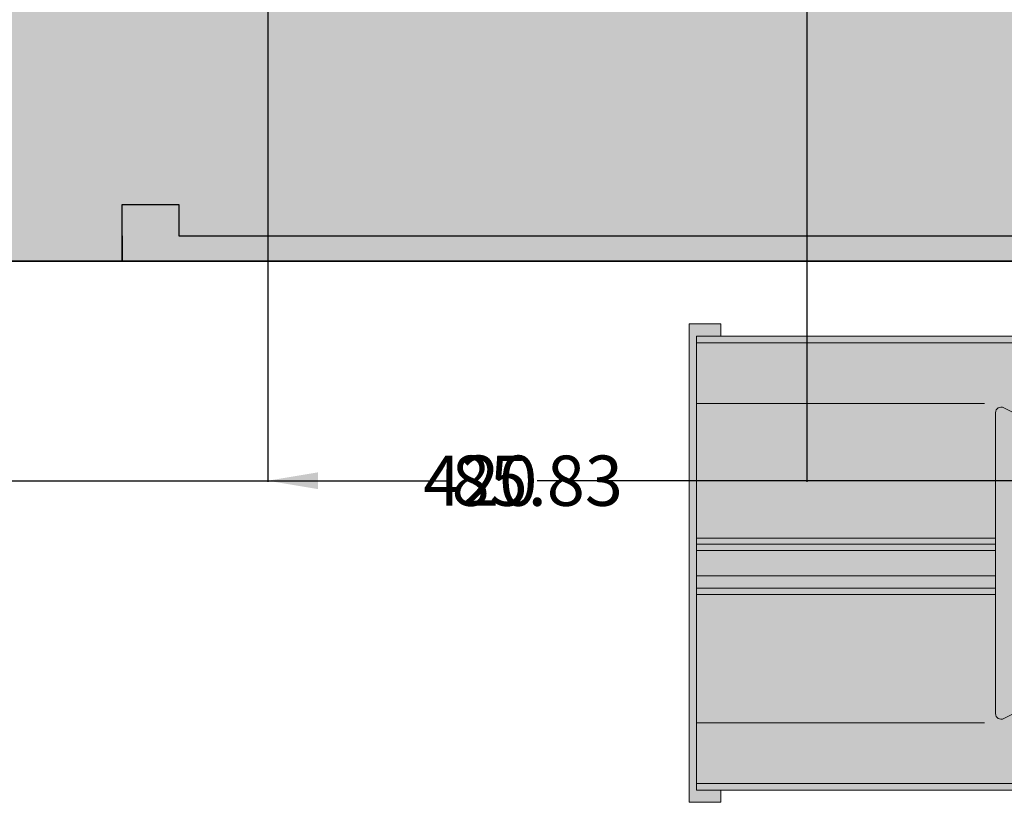
# Model space of a CAD drawing. Units: inches. Extents: x 389 to 971, y 148 to 870.
# Tile 3 of 14: x 565 to 722, y 148 to 273. Entities that reach past the tile are written whole.
import ezdxf

# ---------------------------------------------------------------- set-up
doc = ezdxf.new("R2010")
doc.units = ezdxf.units.IN
doc.header["$MEASUREMENT"] = 0
for name, color, linetype, lineweight in [('A-ANNO-DIMS', 2, 'Continuous', 18), ('C-PROP', 7, 'Continuous', 35), ('C-VEHI', 8, 'Continuous', 13), ('L-GATE', 4, 'Continuous', 25), ('L-GRND-BASE-PATT', 8, 'Continuous', 13), ('L-WALL', 7, 'Continuous', 30)]:
    doc.layers.add(name, color=color, linetype=linetype, lineweight=lineweight)
for name, color, linetype, lineweight, true_color in [('A-WALL-PATT', 18, 'Continuous', 13, 0x000000), ('C-VEHI-PATT', 18, 'Continuous', 13, 0x000000), ('L-GRND-PATT', 39, 'Continuous', 13, 0x603913), ('L-WALL-PATT', 18, 'Continuous', 13, 0x000000)]:
    doc.layers.add(name, color=color, linetype=linetype, lineweight=lineweight, true_color=true_color)
doc.styles.get("Standard").update_dxf_attribs({"font": 'arial.ttf'})
doc.dimstyles.get("Standard").update_dxf_attribs({"dimtxt": 8, "dimasz": 8, "dimexe": 0.18, "dimexo": 0.0625, "dimgap": 0.09, "dimtad": 0, "dimtih": 1, "dimtoh": 1, "dimdec": 0, "dimzin": 0, "dimdsep": 46, "dimlunit": 3, "dimtxsty": 'Standard', "dimcen": 0.09, "dimadec": 0, "dimazin": 0, "dimtfac": 1, "dimtdec": 0, "dimtofl": 0, "dimtmove": 0, "dimatfit": 3, "dimfxl": 1, "dimtolj": 1, "dimtzin": 0, "dimarcsym": 0})

# ---------------------------------------------------------------- blocks, each defined once
blk = doc.blocks.new('*U17')
for p, q in [((1.28, 38.87), (175.66, 38.87)), ((1.28, 28.15), (52.13, 28.15)), ((1.28, -28.15), (52.13, -28.15)), ((1.28, -38.87), (175.66, -38.87))]:
    blk.add_line(p, q)
for points in [[(5.57, 40.01), (5.57, 42.18), (0, 42.18), (0, -42.18), (5.57, -42.18), (5.57, -40.01), (1.28, -40.01), (1.28, 40.01)], [(1.28, 40.01), (175.66, 40.01), (175.66, -40.01), (1.28, -40.01)]]:
    blk.add_lwpolyline(points, close=True)
blk.add_lwpolyline([(55.49, 27.42), (68.59, 20.89, -0.284287), (69.14, 19.99), (69.14, -19.99, -0.284287), (68.59, -20.89), (55.49, -27.42, -0.557284), (54.05, -26.53), (54.05, 26.53, -0.557284)], format="xyb", close=True)
blk = doc.blocks.new('*D44')
at = {"layer": 'A-ANNO-DIMS', "color": 0, "lineweight": -2, "transparency": 16777216}
for p, q in [((428.22, 234.58), (428.22, 199.5)), ((848.22, 234.58), (848.22, 199.5)), ((436.22, 199.68), (629.14, 199.68)), ((840.22, 199.68), (647.29, 199.68))]:
    blk.add_line(p, q, dxfattribs=at)
at = {"layer": 'A-ANNO-DIMS', "color": 0, "transparency": 16777216}
for points in [[(436.22, 201.01), (436.22, 198.34), (428.22, 199.68)], [(840.22, 201.01), (840.22, 198.34), (848.22, 199.68)]]:
    blk.add_solid(points, dxfattribs=at)
at = {"layer": 'Defpoints', "color": 0, "transparency": 16777216}
for p in [(428.22, 234.64), (848.22, 234.64), (848.22, 199.68)]:
    blk.add_point(p, dxfattribs=at)
at = {"layer": 'A-ANNO-DIMS', "color": 0, "transparency": 16777216, "insert": (638.22, 199.68), "char_height": 8, "attachment_point": 5}
blk.add_mtext('\\A1;420', dxfattribs=at)
blk = doc.blocks.new('*D50')
at = {"layer": 'A-ANNO-DIMS', "color": 0, "lineweight": -2, "transparency": 16777216}
for p, q in [((604.39, 294.58), (604.39, 199.5)), ((690.22, 294.58), (690.22, 199.5)), ((612.39, 199.68), (633.71, 199.68)), ((682.22, 199.68), (660.89, 199.68))]:
    blk.add_line(p, q, dxfattribs=at)
at = {"layer": 'A-ANNO-DIMS', "color": 0, "transparency": 16777216}
for points in [[(612.39, 201.01), (612.39, 198.34), (604.39, 199.68)], [(682.22, 201.01), (682.22, 198.34), (690.22, 199.68)]]:
    blk.add_solid(points, dxfattribs=at)
at = {"layer": 'Defpoints', "color": 0, "transparency": 16777216}
for p in [(604.39, 294.64), (690.22, 294.64), (690.22, 199.68)]:
    blk.add_point(p, dxfattribs=at)
at = {"layer": 'A-ANNO-DIMS', "color": 0, "transparency": 16777216, "insert": (647.3, 199.68), "char_height": 8, "attachment_point": 5}
blk.add_mtext('\\A1;85.83', dxfattribs=at)

msp = doc.modelspace()

# ---------------------------------------------------------------- hatches: boundary and pattern name
at = {"layer": 'A-WALL-PATT'}
h = msp.add_hatch(color=256, dxfattribs=at)
h.dxf.hatch_style = 1
h.paths.add_polyline_path([(432.216, 434.6445), (436.3673, 434.6445), (436.3673, 443.6445), (432.216, 443.6445), (432.216, 830.6445), (746.216, 830.6445), (746.216, 823.8175), (755.216, 823.8175), (755.216, 825.6445), (839.216, 825.6445), (839.216, 803.5176), (839.216, 741.6445), (755.216, 741.6445), (755.216, 748.4596), (755.1859, 748.4596), (750.716, 748.4596), (746.216, 748.4596), (746.216, 732.6445), (839.216, 732.6445), (839.216, 600.6445), (708.5171, 600.6445), (708.5171, 596.1445), (708.5171, 591.6445), (794.216, 591.6445), (794.216, 587.4291), (803.216, 587.4291), (803.216, 591.6445), (839.216, 591.6445), (839.216, 466.6012), (803.216, 466.6012), (803.216, 471.0309), (794.216, 471.0309), (794.216, 466.6012), (784.6145, 466.6012), (784.6145, 457.6012), (839.216, 457.6012), (839.216, 447.6445), (839.216, 294.6445), (810.0514, 294.6445), (810.0514, 285.6445), (839.216, 285.6445), (839.216, 238.6445), (590.216, 238.6445), (590.216, 234.6445), (848.216, 234.6445), (848.216, 834.6445), (428.216, 834.6445), (428.216, 234.6445), (437.216, 234.6445), (437.216, 243.6445), (432.216, 243.6445)])
at = {"layer": 'C-VEHI-PATT'}
h = msp.add_hatch(color=256, dxfattribs=at)
h.dxf.hatch_style = 1
h.paths.add_polyline_path([(720.2545, 210.4982), (720.2545, 162.6111, 0.55728405), (721.56, 161.8036), (733.3797, 167.7021, 0.28428722), (733.8792, 168.5096), (733.8792, 204.5997, 0.28428722), (733.3797, 205.4073), (721.56, 211.3058, 0.55728405)], flags=16)
h.paths.add_polyline_path([(672.6289, 151.4772), (723.0515, 151.4772), (723.0515, 157.3254), (736.2011, 165.949, -0.08657677), (736.9651, 166.0823), (754.137, 166.0823, -0.22787473), (755.899, 165.2353), (759.6746, 157.5735), (759.6746, 151.4772), (830.0078, 151.4772), (830.0078, 221.6321), (759.6746, 221.6321), (759.6746, 215.5358), (755.899, 207.8741, -0.22787473), (754.137, 207.0271), (736.9651, 207.0271, -0.08657677), (736.2011, 207.1603), (723.0515, 215.784), (723.0515, 221.6321), (672.6289, 221.6321)])
h.paths.add_polyline_path([(672.6289, 150.445), (676.5048, 150.445), (676.5048, 148.491), (671.4773, 148.491), (671.4773, 224.6184), (676.5048, 224.6184), (676.5048, 222.6644), (672.6289, 222.6644)])
h.paths.add_polyline_path([(735.9785, 205.941), (818.9627, 205.941), (818.9627, 167.1683), (735.9785, 167.1683)], flags=16)
h.paths.add_polyline_path([(727.5014, 158.6254), (736.5823, 164.5807, -0.14613934), (737.0772, 164.7285), (753.9813, 164.7285, -0.29765964), (754.8077, 164.1887), (757.2923, 158.5274, -0.54123619), (757.0857, 158.2111), (727.6252, 158.2111, -0.74498852)], flags=17)
h.paths.add_polyline_path([(727.5014, 214.4839, -0.74498852), (727.6252, 214.8982), (757.0857, 214.8982, -0.54123619), (757.2923, 214.5819), (754.8077, 208.9206, -0.29765964), (753.9813, 208.3808), (737.0772, 208.3808, -0.14613934), (736.5823, 208.5286)], flags=17)
h = msp.add_hatch(color=256, dxfattribs=at)
h.dxf.hatch_style = 1
h.paths.add_polyline_path([(671.4773, 224.6184), (671.4773, 148.491), (676.5048, 148.491), (676.5048, 150.445), (672.6289, 150.445), (672.6289, 222.6644), (676.5048, 222.6644), (676.5048, 224.6184)])
h = msp.add_hatch(color=256, dxfattribs=at)
h.dxf.hatch_style = 1
h.paths.add_polyline_path([(672.6289, 184.5547), (672.6289, 151.4772), (723.0515, 151.4772), (723.0515, 157.3254), (736.2011, 165.949, -0.08657677), (736.9651, 166.0823), (754.137, 166.0823, -0.22787473), (755.899, 165.2353), (759.6746, 157.5735), (759.6746, 151.4772), (830.0078, 151.4772), (830.0078, 221.6321), (759.6746, 221.6321), (759.6746, 215.5358), (755.899, 207.8741, -0.22787473), (754.137, 207.0271), (736.9651, 207.0271, -0.08657677), (736.2011, 207.1603), (723.0515, 215.784), (723.0515, 221.6321), (672.6289, 221.6321), (672.6289, 188.5547), (720.2545, 188.5547), (720.2545, 210.4982, -0.55728405), (721.56, 211.3058), (733.3797, 205.4073, -0.28428722), (733.8792, 204.5997), (733.8792, 168.5096, -0.28428722), (733.3797, 167.7021), (721.56, 161.8036, -0.55728405), (720.2545, 162.6111), (720.2545, 184.5547)], flags=17)
h.paths.add_polyline_path([(672.6289, 151.4772), (723.0515, 151.4772), (723.0515, 157.3254), (736.2011, 165.949, -0.08657677), (736.9651, 166.0823), (754.137, 166.0823, -0.22787473), (755.899, 165.2353), (759.6746, 157.5735), (759.6746, 151.4772), (830.0078, 151.4772), (830.0078, 221.6321), (759.6746, 221.6321), (759.6746, 215.5358), (755.899, 207.8741, -0.22787473), (754.137, 207.0271), (736.9651, 207.0271, -0.08657677), (736.2011, 207.1603), (723.0515, 215.784), (723.0515, 221.6321), (672.6289, 221.6321)], flags=17)
h.paths.add_polyline_path([(672.6289, 150.445), (676.5048, 150.445), (676.5048, 148.491), (671.4773, 148.491), (671.4773, 224.6184), (676.5048, 224.6184), (676.5048, 222.6644), (672.6289, 222.6644)])
h.paths.add_polyline_path([(720.2545, 210.4982, -0.55728405), (721.56, 211.3058), (733.3797, 205.4073, -0.28428722), (733.8792, 204.5997), (733.8792, 168.5096, -0.28428722), (733.3797, 167.7021), (721.56, 161.8036, -0.55728405), (720.2545, 162.6111)], flags=0)
h.paths.add_polyline_path([(727.5014, 158.6254), (736.5823, 164.5807, -0.14613934), (737.0772, 164.7285), (753.9813, 164.7285, -0.29765964), (754.8077, 164.1887), (757.2923, 158.5274, -0.54123619), (757.0857, 158.2111), (727.6252, 158.2111, -0.74498852)], flags=0)
h = msp.add_hatch(color=256, dxfattribs=at)
h.dxf.hatch_style = 1
h.paths.add_polyline_path([(671.4773, 148.491), (676.5048, 148.491), (676.5048, 150.445), (672.6289, 150.445), (672.6289, 222.6644), (676.5048, 222.6644), (676.5048, 224.6184), (671.4773, 224.6184)])
h = msp.add_hatch(color=256, dxfattribs=at)
h.dxf.hatch_style = 1
h.paths.add_polyline_path([(723.0515, 221.6321), (723.0515, 215.784), (736.2011, 207.1603, 0.08657677), (736.9651, 207.0271), (754.137, 207.0271, 0.22787473), (755.899, 207.8741), (759.6746, 215.5358), (759.6746, 221.6321)], flags=16)
h.paths.add_polyline_path([(672.6289, 222.6644), (672.6289, 151.4772), (723.0515, 151.4772), (723.0515, 157.3254), (736.2011, 165.949, -0.08657677), (736.9651, 166.0823), (754.137, 166.0823, -0.22787473), (755.899, 165.2353), (759.6746, 157.5735), (759.6746, 151.4772), (830.0078, 151.4772), (830.0078, 222.6644)])
h = msp.add_hatch(color=256, dxfattribs=at)
h.dxf.hatch_style = 1
h.paths.add_polyline_path([(723.0515, 221.6321), (723.0515, 222.6644), (672.6289, 222.6644), (672.6289, 221.6321)])
h = msp.add_hatch(color=256, dxfattribs=at)
h.dxf.hatch_style = 1
h.paths.add_polyline_path([(733.8792, 204.5997, 0.28428722), (733.3797, 205.4073), (721.56, 211.3058, 0.55728405), (720.2545, 210.4982), (720.2545, 162.6111, 0.55728405), (721.56, 161.8036), (733.3797, 167.7021, 0.28428722), (733.8792, 168.5096)])
h = msp.add_hatch(color=256, dxfattribs=at)
h.dxf.hatch_style = 1
h.paths.add_polyline_path([(720.2545, 162.6111, 0.55728405), (721.56, 161.8036), (733.3797, 167.7021, 0.28428722), (733.8792, 168.5096), (733.8792, 204.5997, 0.28428722), (733.3797, 205.4073), (721.56, 211.3058, 0.55728405), (720.2545, 210.4982)])
h = msp.add_hatch(color=256, dxfattribs=at)
h.dxf.hatch_style = 1
h.paths.add_polyline_path([(733.8792, 204.5997, 0.28428722), (733.3797, 205.4073), (721.56, 211.3058, 0.55728405), (720.2545, 210.4982), (720.2545, 162.6111, 0.55728405), (721.56, 161.8036), (733.3797, 167.7021, 0.28428722), (733.8792, 168.5096)])
h = msp.add_hatch(color=256, dxfattribs=at)
h.dxf.hatch_style = 1
h.paths.add_polyline_path([(672.6289, 190.5547), (672.6289, 189.5547), (720.2545, 189.5547), (720.2545, 190.5547)])
h = msp.add_hatch(color=256, dxfattribs=at)
h.dxf.hatch_style = 1
h.paths.add_polyline_path([(672.6289, 182.5547), (672.6289, 181.5547), (720.2545, 181.5547), (720.2545, 182.5547)])
h = msp.add_hatch(color=256, dxfattribs=at)
h.dxf.hatch_style = 1
h.paths.add_polyline_path([(723.0515, 150.445), (723.0515, 151.4772), (672.6289, 151.4772), (672.6289, 150.445)])
at = {"layer": 'L-GRND-BASE-PATT'}
h = msp.add_hatch(color=256, dxfattribs=at)
h.dxf.hatch_style = 1
edge = h.paths.add_edge_path(flags=16)
edge.add_ellipse((8782.0026, 354.2473), major_axis=(-8296.9493, 0), ratio=0.84230387, start_angle=-0.09022909, end_angle=0.38386678, ccw=False)
edge.add_ellipse((485.0533, 368.2895), major_axis=(-1.1591, 0), ratio=0.84230387, start_angle=0, end_angle=90, ccw=False)
edge.add_line((483.8943, 368.2895), (483.8943, 387.6039))
edge.add_ellipse((485.0533, 387.2466), major_axis=(1.1591, 0), ratio=0.84230387, start_angle=90, end_angle=180, ccw=False)
edge.add_line((485.0533, 388.2229), (485.5047, 388.2229))
edge.add_ellipse((898.8202, 372.4897), major_axis=(413.7374, 0), ratio=0.84230387, start_angle=176.349572, end_angle=177.82005, ccw=False)
edge.add_ellipse((535.9119, 196.3855), major_axis=(-245.3972, 0), ratio=0.84230387, start_angle=-77.874034, end_angle=-76.219471, ccw=False)
edge.add_ellipse((535.9119, 201.7547), major_axis=(239.1274, 0), ratio=0.84230387, start_angle=100.209539, end_angle=102.444627, ccw=False)
edge.add_ellipse((473.3139, 564.9222), major_axis=(196.5637, 0), ratio=0.84230387, start_angle=-80.743434, end_angle=-77.445067)
edge.add_line((509.5535, 402.1941), (514.3535, 404.8483))
edge.add_line((514.3535, 404.8483), (514.3535, 404.7972))
edge.add_ellipse((514.3535, 404.2644), major_axis=(0.5795, 0), ratio=0.84230387, start_angle=52.06687, end_angle=90, ccw=False)
edge.add_line((514.6716, 404.6725), (519.1535, 402.1941))
edge.add_ellipse((555.3932, 564.9222), major_axis=(-196.5637, 0), ratio=0.84230387, start_angle=77.445067, end_angle=80.743434)
edge.add_ellipse((492.7951, 201.7547), major_axis=(239.1274, 0), ratio=0.84230387, start_angle=77.555373, end_angle=79.790461, ccw=False)
edge.add_ellipse((492.7951, 196.3855), major_axis=(245.3972, 0), ratio=0.84230387, start_angle=76.219471, end_angle=77.874034, ccw=False)
edge.add_ellipse((129.8868, 372.4897), major_axis=(-413.7374, 0), ratio=0.84230387, start_angle=182.17995, end_angle=183.650428, ccw=False)
edge.add_line((543.2023, 388.2229), (544.0779, 388.2229))
edge.add_ellipse((543.6537, 387.2466), major_axis=(-1.1591, 0), ratio=0.84230387, start_angle=180, end_angle=270, ccw=False)
edge.add_line((544.8128, 387.2466), (544.8128, 367.9322))
edge.add_ellipse((543.6537, 368.2895), major_axis=(1.1591, 0), ratio=0.84230387, start_angle=270, end_angle=360, ccw=False)
edge.add_ellipse((-7753.2956, 354.2473), major_axis=(-8296.9493, 0), ratio=0.84230387, start_angle=179.61613322, end_angle=180.09022909, ccw=False)
edge.add_line((543.3912, 298.6608), (544.0779, 298.6608))
edge.add_ellipse((543.6537, 297.6845), major_axis=(1.1591, 0), ratio=0.84230387, start_angle=0, end_angle=90, ccw=False)
edge.add_line((544.8128, 297.6845), (544.8128, 278.3701))
edge.add_ellipse((543.6537, 278.7275), major_axis=(-1.1591, 0), ratio=0.84230387, start_angle=90, end_angle=180, ccw=False)
edge.add_line((543.6537, 277.7512), (543.1566, 277.7512))
edge.add_ellipse((-7753.2956, 354.2473), major_axis=(-8296.9493, 0), ratio=0.84230387, start_angle=179.3813568, end_angle=179.47172853, ccw=False)
edge.add_ellipse((542.4236, 263.2763), major_axis=(-1.7386, 0), ratio=0.84230387, start_angle=179.371763, end_angle=248.464757, ccw=False)
edge.add_ellipse((-7753.8751, 354.2473), major_axis=(-8298.7403, 0), ratio=0.842303866, start_angle=179.35344592, end_angle=179.3717628, ccw=False)
edge.add_ellipse((540.0116, 260.6509), major_axis=(-4.1092, 0), ratio=0.84230387, start_angle=90, end_angle=179.353446, ccw=False)
edge.add_line((540.0116, 257.1897), (488.6954, 257.1897))
edge.add_ellipse((488.6954, 260.6509), major_axis=(4.1092, 0), ratio=0.84230387, start_angle=180.646554, end_angle=270, ccw=False)
edge.add_ellipse((8782.5821, 354.2473), major_axis=(-8298.7403, 0), ratio=0.842303872, start_angle=0.62823723, end_angle=0.64655411, ccw=False)
edge.add_ellipse((486.2834, 263.2763), major_axis=(-1.7386, 0), ratio=0.84230387, start_angle=-68.464756, end_angle=0.628237, ccw=False)
edge.add_ellipse((8782.0026, 354.2473), major_axis=(-8296.9493, 0), ratio=0.84230387, start_angle=0.52827147, end_angle=0.6465541, ccw=False)
edge.add_line((485.5504, 277.7512), (484.6291, 277.7512))
edge.add_ellipse((485.0533, 278.7275), major_axis=(-1.1591, 0), ratio=0.84230387, start_angle=0, end_angle=90, ccw=False)
edge.add_line((483.8943, 278.7275), (483.8943, 298.0418))
edge.add_ellipse((485.0533, 297.6845), major_axis=(1.1591, 0), ratio=0.84230387, start_angle=90, end_angle=180, ccw=False)
edge = h.paths.add_edge_path(flags=0)
edge.add_ellipse((8782.0026, 354.2473), major_axis=(-8295.7902, 0), ratio=0.84230387, start_angle=0.05559431, end_angle=0.37776419, ccw=False)
edge.add_line((486.2179, 346.1978), (489.3905, 335.8384))
edge.add_ellipse((3386.0114, 329.7263), major_axis=(-2896.63, 0), ratio=0.84230387, start_angle=-0.1208974, end_angle=0.3640763)
edge.add_line((489.4638, 311.3204), (486.4666, 299.5521))
edge = h.paths.add_edge_path(flags=0)
edge.add_ellipse((514.3535, 391.3731), major_axis=(-115.1513, 0), ratio=0.84230387, start_angle=76.401865, end_angle=103.598135)
edge.add_line((537.3428, 296.3333), (537.3428, 281.5897))
edge.add_ellipse((514.3535, 376.6295), major_axis=(-115.1513, 0), ratio=0.84230387, start_angle=76.401865, end_angle=103.598135, ccw=False)
edge.add_line((491.3643, 281.5897), (491.3643, 296.3333))
edge = h.paths.add_edge_path(flags=0)
edge.add_line((491.3643, 337.0752), (489.653, 349.9016))
edge.add_ellipse((510.1338, 298.7862), major_axis=(64.0481, 0), ratio=0.84230387, start_angle=94.277421, end_angle=111.834954, ccw=False)
edge.add_line((506.1068, 352.6274), (522.6002, 352.6274))
edge.add_ellipse((518.5732, 298.7862), major_axis=(64.0481, 0), ratio=0.84230387, start_angle=68.165046, end_angle=85.722579, ccw=False)
edge.add_line((539.0541, 349.9016), (537.3428, 337.0752))
edge.add_ellipse((516.5462, 287.5825), major_axis=(62.3305, 0), ratio=0.84230387, start_angle=67.208085, end_angle=85.12993)
edge.add_line((521.008, 339.949), (507.699, 339.949))
edge.add_ellipse((512.1609, 287.5825), major_axis=(62.3305, 0), ratio=0.84230387, start_angle=94.87007, end_angle=112.791915)
edge = h.paths.add_edge_path(flags=0)
edge.add_ellipse((493.6824, 273.9439), major_axis=(-2.3182, 0), ratio=0.84230387, start_angle=-90, end_angle=0, ccw=False)
edge.add_line((493.6824, 275.8965), (535.3743, 275.8965))
edge.add_ellipse((535.0246, 273.9439), major_axis=(2.3182, 0), ratio=0.84230387, start_angle=0, end_angle=90, ccw=False)
edge.add_line((537.3428, 273.9439), (537.3428, 258.6983))
edge.add_line((537.3428, 258.6983), (540.5912, 258.6983))
edge.add_ellipse((540.5912, 260.6509), major_axis=(-2.3182, 0), ratio=0.84230387, start_angle=90, end_angle=179.353446)
edge.add_line((540.5912, 258.6983), (487.7691, 258.6983))
edge.add_ellipse((488.1158, 260.6509), major_axis=(2.3182, 0), ratio=0.84230387, start_angle=180.646554, end_angle=270)
edge.add_line((488.1158, 258.6983), (491.3643, 258.6983))
edge.add_line((491.3643, 258.6983), (491.3643, 274.2384))
h.paths.add_polyline_path([(746.1376, 327.3223), (750.14, 327.3223), (750.14, 326.2831), (798.1694, 326.2831), (798.1694, 327.3223), (802.1718, 327.3223), (802.1718, 309.9784, -0.19047621), (746.1376, 309.9784)], flags=16)
h.paths.add_polyline_path([(782.1596, 313.5685), (782.1596, 309.0415, -0.04962821), (766.1498, 309.0415), (766.1498, 313.5685)], flags=0)
h.paths.add_polyline_path([(755.1859, 344.9352), (755.1859, 373.9163), (788.1244, 373.9163), (788.1244, 344.9352)], flags=16)
h.paths.add_polyline_path([(757.1859, 346.9352), (757.1859, 371.9163), (786.1244, 371.9163), (786.1244, 346.9352)], flags=0)
h.paths.add_polyline_path([(803.6446, 338.4879), (803.6446, 342.4903), (804.6838, 342.4903), (804.6838, 390.5197), (803.6446, 390.5197), (803.6446, 394.5221), (820.9885, 394.5221, -0.19047621), (820.9885, 338.4879)], flags=16)
h.paths.add_polyline_path([(806.8707, 326.6963), (806.4254, 327.1416), (806.4724, 326.6297)], flags=16)
h.paths.add_polyline_path([(822.0328, 317.4008), (822.1942, 317.8933), (821.5626, 317.9885)], flags=16)
h.paths.add_polyline_path([(817.3984, 358.5001), (817.3984, 374.5099), (821.9254, 374.5099, -0.04962821), (821.9254, 358.5001)], flags=0)
h.paths.add_polyline_path([(808.1446, 418.9737), (808.2247, 418.5632), (808.5395, 418.5787)], flags=16)
h.paths.add_polyline_path([(820.3159, 412.669), (820.4772, 413.1615), (819.8457, 413.2568)], flags=16)
h.paths.add_polyline_path([(466.3155, 235.5246), (517.3807, 235.5246), (517.3807, 244.4269), (466.3155, 244.4269)], flags=24)
h.paths.add_polyline_path([(739.8737, 256.2), (815.404, 256.2), (815.404, 265.3454), (739.8737, 265.3454)], flags=24)
h.paths.add_polyline_path([(750.6082, 393.6667), (791.5681, 393.6667), (791.5681, 412.3933), (750.6082, 412.3933)], flags=24)
h.paths.add_polyline_path([(438.9631, 410.0619), (484.6204, 410.0619), (484.6204, 429.1217), (438.9631, 429.1217)], flags=24)
edge = h.paths.add_edge_path()
edge.add_line((839.216, 285.6445), (611.8787, 285.6445))
edge.add_line((611.8787, 285.6445), (604.387, 285.6445))
edge.add_line((604.387, 285.6445), (595.387, 285.6445))
edge.add_line((595.387, 285.6445), (595.387, 370.1554))
edge.add_line((595.387, 370.1554), (604.0817, 370.1554))
edge.add_line((604.0817, 370.1554), (604.0817, 371.3788))
edge.add_line((604.0817, 371.3788), (632.0195, 371.3788))
edge.add_arc((604.0817, 370.1554), 27.9645, 2.507491, 90)
edge.add_line((604.0817, 398.1199), (599.887, 398.1652))
edge.add_line((599.887, 398.1652), (604.4225, 398.1652))
edge.add_arc((604.4225, 428.4021), 30.2369, 270, 357.492509)
edge.add_line((634.6305, 427.0792), (604.4225, 427.0792))
edge.add_line((604.4225, 427.0792), (604.4225, 428.4021))
edge.add_line((604.4225, 428.4021), (599.887, 428.4021))
edge.add_line((599.887, 428.4021), (595.387, 428.4021))
edge.add_line((595.387, 428.4021), (595.387, 434.6445))
edge.add_line((595.387, 434.6445), (585.0791, 434.6445))
edge.add_line((585.0791, 434.6445), (540.3922, 434.6445))
edge.add_line((540.3922, 434.6445), (526.7125, 434.6445))
edge.add_line((526.7125, 434.6445), (488.4095, 434.6445))
edge.add_line((488.4095, 434.6445), (432.216, 434.6445))
edge.add_line((432.216, 434.6445), (432.216, 243.6445))
edge.add_line((432.216, 243.6445), (437.216, 243.6445))
edge.add_line((437.216, 243.6445), (437.216, 234.6445))
edge.add_line((437.216, 234.6445), (581.216, 234.6445))
edge.add_line((581.216, 234.6445), (581.216, 238.6445))
edge.add_line((581.216, 238.6445), (581.216, 243.6445))
edge.add_line((581.216, 243.6445), (590.216, 243.6445))
edge.add_line((590.216, 243.6445), (590.216, 238.6445))
edge.add_line((590.216, 238.6445), (839.216, 238.6445))
edge.add_line((839.216, 238.6445), (839.216, 285.6445))
at = {"layer": 'L-GRND-PATT'}
h = msp.add_hatch(dxfattribs=at)
h.set_pattern_fill('EARTH', color=256, angle=45)
h.set_pattern_definition([(45, (0, 0), (0, 8.980256), [6.35, -6.35]), (45, (-1.684, 1.684), (0, 8.980256), [6.35, -6.35]), (45, (-3.3676, 3.3676), (0, 8.980256), [6.35, -6.35]), (135, (-3.3676, 4.49), (-8.980256, 0), [6.35, -6.35]), (135, (-1.684, 6.174), (-8.980256, 0), [6.35, -6.35]), (135, (0, 7.858), (-8.980256, 0), [6.35, -6.35])])
h.paths.add_polyline_path([(432.216, 243.6445), (437.216, 243.6445), (437.216, 234.6445), (581.216, 234.6445), (581.216, 238.6445), (581.216, 243.6445), (590.216, 243.6445), (590.216, 238.6445), (839.216, 238.6445), (839.216, 285.6445), (810.0514, 285.6445), (733.8057, 285.6445), (684.2434, 285.6445), (611.8787, 285.6445), (604.387, 285.6445), (595.387, 285.6445), (595.387, 370.1554), (604.0817, 370.1554), (604.0817, 371.3788), (632.0195, 371.3788, 0.40145271), (604.0817, 398.1199), (599.887, 398.1652), (604.4225, 398.1652, 0.40145271), (634.6305, 427.0792), (604.4225, 427.0792), (604.4225, 428.4021), (599.887, 428.4021), (595.387, 428.4021), (595.387, 434.6445), (585.0791, 434.6445), (540.3922, 434.6445), (526.7125, 434.6445), (488.4095, 434.6445), (432.216, 434.6445)])
edge = h.paths.add_edge_path(flags=16)
edge.add_line((483.8943, 278.7275), (483.8943, 298.2564))
edge.add_ellipse((485.0533, 297.6845), major_axis=(1.1591, 0), ratio=0.84230387, start_angle=90, end_angle=180, ccw=False)
edge.add_ellipse((8782.0026, 354.2473), major_axis=(-8296.9493, 0), ratio=0.84230387, start_angle=-0.09022909, end_angle=0.38386678, ccw=False)
edge.add_ellipse((485.0533, 368.2895), major_axis=(-1.1591, 0), ratio=0.84230387, start_angle=0, end_angle=90, ccw=False)
edge.add_line((483.8943, 368.2895), (483.8943, 387.8185))
edge.add_ellipse((485.0533, 387.2466), major_axis=(1.1591, 0), ratio=0.84230387, start_angle=90, end_angle=180, ccw=False)
edge.add_ellipse((898.8202, 372.4897), major_axis=(413.7374, 0), ratio=0.84230387, start_angle=176.349572, end_angle=177.82005, ccw=False)
edge.add_ellipse((535.9119, 196.3855), major_axis=(-245.3972, 0), ratio=0.84230387, start_angle=-77.874034, end_angle=-76.219471, ccw=False)
edge.add_ellipse((535.9119, 201.7547), major_axis=(239.1274, 0), ratio=0.84230387, start_angle=100.209539, end_angle=102.444627, ccw=False)
edge.add_ellipse((473.3139, 564.9222), major_axis=(196.5637, 0), ratio=0.84230387, start_angle=-80.743434, end_angle=-77.445067)
edge.add_line((509.5535, 402.1941), (514.3535, 404.8483))
edge.add_line((514.3535, 404.8483), (519.1535, 402.1941))
edge.add_ellipse((555.3932, 564.9222), major_axis=(-196.5637, 0), ratio=0.84230387, start_angle=77.445067, end_angle=80.743434)
edge.add_ellipse((492.7951, 201.7547), major_axis=(239.1274, 0), ratio=0.84230387, start_angle=77.555373, end_angle=79.790461, ccw=False)
edge.add_ellipse((492.7951, 196.3855), major_axis=(245.3972, 0), ratio=0.84230387, start_angle=76.219471, end_angle=77.874034, ccw=False)
edge.add_ellipse((129.8868, 372.4897), major_axis=(-413.7374, 0), ratio=0.84230387, start_angle=182.17995, end_angle=183.650428, ccw=False)
edge.add_line((543.2023, 388.2229), (544.3327, 388.2229))
edge.add_ellipse((543.6537, 387.2466), major_axis=(-1.1591, 0), ratio=0.84230387, start_angle=180, end_angle=270, ccw=False)
edge.add_line((544.8128, 387.2466), (544.8128, 367.7176))
edge.add_ellipse((543.6537, 368.2895), major_axis=(1.1591, 0), ratio=0.84230387, start_angle=270, end_angle=360, ccw=False)
edge.add_ellipse((-7753.2956, 354.2473), major_axis=(-8296.9493, 0), ratio=0.84230387, start_angle=179.61613322, end_angle=180.09022909, ccw=False)
edge.add_ellipse((543.6537, 297.6845), major_axis=(1.1591, 0), ratio=0.84230387, start_angle=0, end_angle=90, ccw=False)
edge.add_line((544.8128, 297.6845), (544.8128, 278.1556))
edge.add_ellipse((543.6537, 278.7275), major_axis=(-1.1591, 0), ratio=0.84230387, start_angle=90, end_angle=180, ccw=False)
edge.add_ellipse((-7753.2956, 354.2473), major_axis=(-8296.9493, 0), ratio=0.84230387, start_angle=179.3813568, end_angle=179.47172853, ccw=False)
edge.add_ellipse((542.4236, 263.2763), major_axis=(-1.7386, 0), ratio=0.84230387, start_angle=179.371763, end_angle=248.464757, ccw=False)
edge.add_ellipse((-7753.8751, 354.2473), major_axis=(-8298.7403, 0), ratio=0.842303866, start_angle=179.35344592, end_angle=179.3717628, ccw=False)
edge.add_ellipse((540.0116, 260.6509), major_axis=(-4.1092, 0), ratio=0.84230387, start_angle=90, end_angle=179.353446, ccw=False)
edge.add_line((540.0116, 257.1897), (488.0808, 257.1897))
edge.add_ellipse((488.6954, 260.6509), major_axis=(4.1092, 0), ratio=0.84230387, start_angle=180.646554, end_angle=270, ccw=False)
edge.add_ellipse((8782.5821, 354.2473), major_axis=(-8298.7403, 0), ratio=0.842303872, start_angle=0.62823723, end_angle=0.64655411, ccw=False)
edge.add_ellipse((486.2834, 263.2763), major_axis=(-1.7386, 0), ratio=0.84230387, start_angle=-68.464756, end_angle=0.628237, ccw=False)
edge.add_ellipse((8782.0026, 354.2473), major_axis=(-8296.9493, 0), ratio=0.84230387, start_angle=0.52827147, end_angle=0.6465541, ccw=False)
edge.add_line((485.5504, 277.7512), (484.3744, 277.7512))
edge.add_ellipse((485.0533, 278.7275), major_axis=(-1.1591, 0), ratio=0.84230387, start_angle=0, end_angle=90, ccw=False)
edge = h.paths.add_edge_path(flags=0)
edge.add_ellipse((488.1158, 260.6509), major_axis=(2.3182, 0), ratio=0.84230387, start_angle=180.646554, end_angle=270)
edge.add_line((488.1158, 258.6983), (491.3643, 258.6983))
edge.add_line((491.3643, 258.6983), (491.3643, 274.4686))
edge.add_ellipse((493.6824, 273.9439), major_axis=(-2.3182, 0), ratio=0.84230387, start_angle=-90, end_angle=0, ccw=False)
edge.add_line((493.6824, 275.8965), (535.6476, 275.8965))
edge.add_ellipse((535.0246, 273.9439), major_axis=(2.3182, 0), ratio=0.84230387, start_angle=0, end_angle=90, ccw=False)
edge.add_line((537.3428, 273.9439), (537.3428, 258.6983))
edge.add_line((537.3428, 258.6983), (541.2086, 258.6983))
edge.add_ellipse((540.5912, 260.6509), major_axis=(-2.3182, 0), ratio=0.84230387, start_angle=90, end_angle=179.353446, ccw=False)
edge.add_line((540.5912, 258.6983), (487.4984, 258.6983))
edge = h.paths.add_edge_path(flags=0)
edge.add_line((491.3643, 281.5897), (491.3643, 296.3333))
edge.add_ellipse((514.3535, 391.3731), major_axis=(-115.1513, 0), ratio=0.84230387, start_angle=76.401865, end_angle=103.598135)
edge.add_line((537.3428, 296.3333), (537.3428, 281.5897))
edge.add_ellipse((514.3535, 376.6295), major_axis=(-115.1513, 0), ratio=0.84230387, start_angle=76.401865, end_angle=103.598135, ccw=False)
edge = h.paths.add_edge_path(flags=0)
edge.add_ellipse((8782.0026, 354.2473), major_axis=(-8295.7902, 0), ratio=0.84230387, start_angle=0.05559431, end_angle=0.37776419, ccw=False)
edge.add_line((486.2179, 346.1978), (489.3905, 335.8384))
edge.add_ellipse((3386.0114, 329.7263), major_axis=(-2896.63, 0), ratio=0.84230387, start_angle=-0.1208974, end_angle=0.3640763)
edge.add_line((489.4638, 311.3204), (486.4666, 299.5521))
edge = h.paths.add_edge_path(flags=0)
edge.add_line((491.3643, 337.0752), (489.653, 349.9016))
edge.add_ellipse((510.1338, 298.7862), major_axis=(64.0481, 0), ratio=0.84230387, start_angle=94.277421, end_angle=111.834954, ccw=False)
edge.add_line((506.1068, 352.6274), (522.6002, 352.6274))
edge.add_ellipse((518.5732, 298.7862), major_axis=(64.0481, 0), ratio=0.84230387, start_angle=68.165046, end_angle=85.722579, ccw=False)
edge.add_line((539.0541, 349.9016), (537.3428, 337.0752))
edge.add_ellipse((516.5462, 287.5825), major_axis=(62.3305, 0), ratio=0.84230387, start_angle=67.208085, end_angle=85.12993)
edge.add_line((521.008, 339.949), (507.699, 339.949))
edge.add_ellipse((512.1609, 287.5825), major_axis=(62.3305, 0), ratio=0.84230387, start_angle=94.87007, end_angle=112.791915)
h.paths.add_polyline_path([(466.3155, 235.5246), (517.3807, 235.5246), (517.3807, 244.4269), (466.3155, 244.4269)], flags=24)
h.paths.add_polyline_path([(739.8737, 256.2), (815.404, 256.2), (815.404, 265.3454), (739.8737, 265.3454)], flags=24)
h.paths.add_polyline_path([(438.9631, 410.0619), (484.6204, 410.0619), (484.6204, 429.1217), (438.9631, 429.1217)], flags=24)
at = {"layer": 'L-WALL-PATT'}
h = msp.add_hatch(color=256, dxfattribs=at)
h.dxf.hatch_style = 1
h.paths.add_polyline_path([(581.216, 243.6445), (581.216, 234.6445), (590.216, 234.6445), (590.216, 243.6445)])

# ---------------------------------------------------------------- linework, layer by layer
at = {"layer": 'C-PROP'}
msp.add_line((428.216, 234.6445), (848.216, 234.6445), dxfattribs=at)
at = {"layer": 'C-VEHI'}
for p, q in [((720.2545, 190.5547), (672.6289, 190.5547)), ((720.2545, 189.5547), (720.2545, 190.5547)), ((672.6289, 188.5547), (672.6289, 189.5547)), ((672.6289, 189.5547), (720.2545, 189.5547)), ((720.2545, 188.5547), (672.6289, 188.5547)), ((672.6289, 188.5547), (672.6289, 184.5547)), ((720.2545, 186.5547), (720.2545, 188.5547)), ((672.6289, 184.5547), (720.2545, 184.5547)), ((672.6289, 184.5547), (672.6289, 182.5547)), ((672.6289, 182.5547), (720.2545, 182.5547)), ((720.2545, 182.5547), (720.2545, 181.5547)), ((720.2545, 181.5547), (672.6289, 181.5547))]:
    msp.add_line(p, q, dxfattribs=at)
at = {"layer": 'L-GATE'}
msp.add_line((437.216, 234.6445), (581.216, 234.6445), dxfattribs=at)
at = {"layer": 'L-WALL'}
for p, q in [((581.216, 234.6445), (581.216, 243.6445)), ((581.216, 243.6445), (590.216, 243.6445)), ((590.216, 243.6445), (590.216, 238.6445)), ((581.216, 238.6445), (581.216, 234.6445)), ((590.216, 238.6445), (839.216, 238.6445))]:
    msp.add_line(p, q, dxfattribs=at)

# ---------------------------------------------------------------- block references
at = {"layer": 'C-VEHI', "xscale": 0.902504869863545, "yscale": 0.902504869863545, "zscale": 0.902504869863545}
msp.add_blockref('*U17', (671.4773, 186.5547), dxfattribs=at)

# ---------------------------------------------------------------- dimensions: what is measured, and where the dimension line sits
at = {"layer": 'A-ANNO-DIMS'}
for base, p1, p2, override, picture, middle in [((690.216, 199.6753), (604.387, 294.6445), (690.216, 294.6445), {"dimdec": 2, "dimlfac": 1, "dimrnd": 0, "dimzin": 0, "dimdsep": 46, "dimlunit": 2}, '*D50', (647.3015, 199.6753)), ((848.216, 199.6753), (428.216, 234.6445), (848.216, 234.6445), {"dimdec": 0, "dimlfac": 1, "dimrnd": 0, "dimzin": 0, "dimdsep": 46, "dimlunit": 2}, '*D44', (638.216, 199.6753))]:
    dim = msp.add_linear_dim(base=base, p1=p1, p2=p2, dimstyle='Standard', override=override, dxfattribs=at)
    dim.commit()
    dim.dimension.update_dxf_attribs({"geometry": picture, "text_midpoint": middle})

doc.saveas('drawing.dxf')
